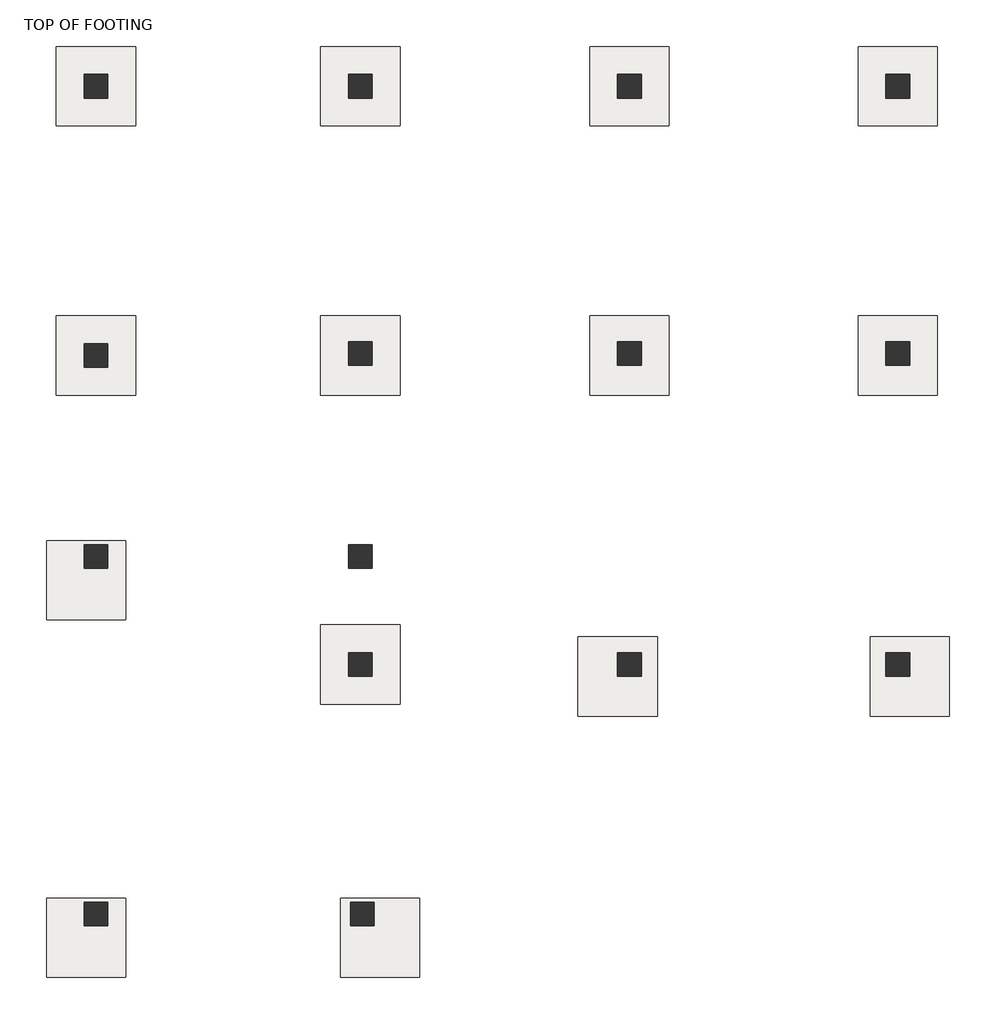
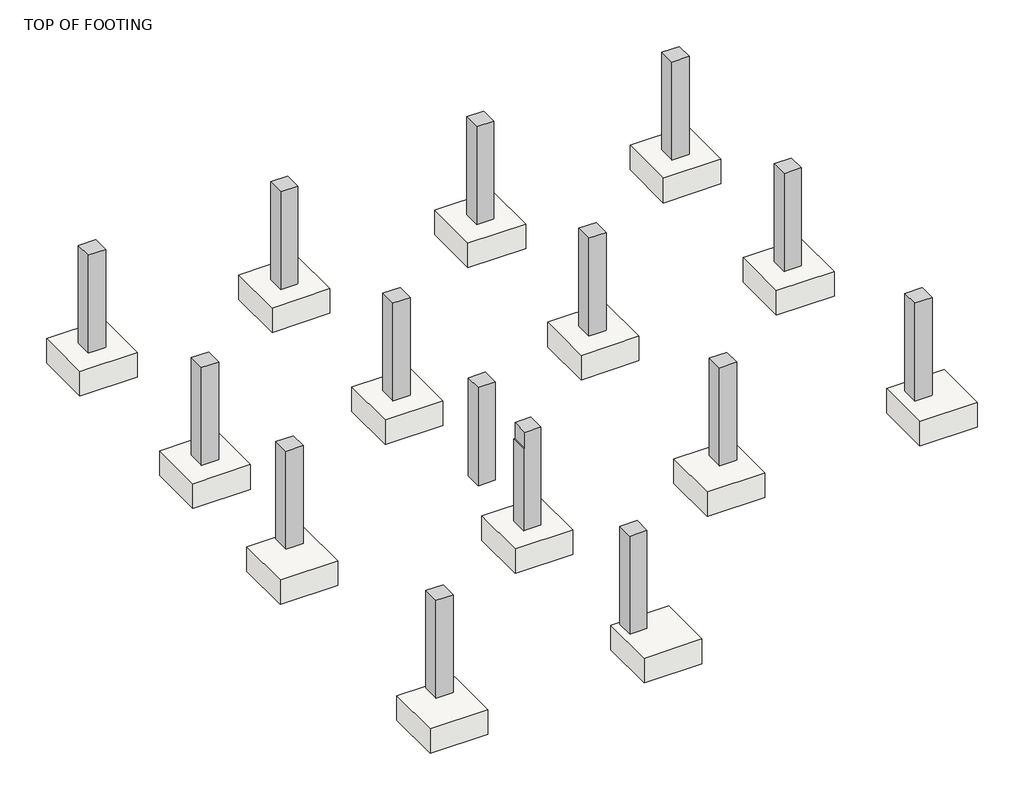
# One storey: 15 columns, 14 slabs.
"""IFC4 building model written with IfcOpenShell, lengths in millimetres."""

from ifc_helpers import new_model, si_unit, frame, origin, place, context, project, spatial, polyline, outline, extrude, faceted_brep, transform, mapped, element, save
from components import slab_21579c01

model = new_model("IFC4")

# Units and contexts
model_context = context("Model", 3, world=origin())
ifc_project = project(units=[si_unit("LENGTHUNIT", "METRE", prefix="MILLI")], contexts=[model_context])

# Site, building, storey
site = spatial("IfcSite", under=ifc_project)
building = spatial("IfcBuilding", under=site)
storey = spatial("IfcBuildingStorey", under=building, Name="TOP OF FOOTING", Elevation=-1828.8)

# Columns
placement = place(None, origin())
element("IfcColumn", 1, ObjectType="Concrete-Rectangular-Column : 12\" X 12\" COLUMN", at=placement, inside=storey, context=model_context, shape_type="SweptSolid", body=[
    extrude(outline(polyline([(-11339.0293601, -2564.0747117), (-11339.0293601, -2868.8747117), (-11643.8293601, -2868.8747117), (-11643.8293601, -2564.0747117), (-11339.0293601, -2564.0747117)])), frame((0.0, 0.0, -1828.8), z_axis=(0.0, 0.0, 1.0), x_axis=(1.0, 0.0, 0.0)), (0.0, 0.0, 1.0), 1828.8),
])
element("IfcColumn", 2, ObjectType="Concrete-Rectangular-Column : 12\" X 12\" COLUMN", at=placement, inside=storey, context=model_context, shape_type="SweptSolid", body=[
    extrude(outline(polyline([(-7946.7270642, -2564.0747117), (-7946.7270642, -2868.8747117), (-8251.5270642, -2868.8747117), (-8251.5270642, -2564.0747117), (-7946.7270642, -2564.0747117)])), frame((0.0, 0.0, -1828.8), z_axis=(0.0, 0.0, 1.0), x_axis=(1.0, 0.0, 0.0)), (0.0, 0.0, 1.0), 1828.8),
])
element("IfcColumn", 3, ObjectType="Concrete-Rectangular-Column : 12\" X 12\" COLUMN", at=placement, inside=storey, context=model_context, shape_type="SweptSolid", body=[
    extrude(outline(polyline([(-4492.3270642, -2564.0747117), (-4492.3270642, -2868.8747117), (-4797.1270642, -2868.8747117), (-4797.1270642, -2564.0747117), (-4492.3270642, -2564.0747117)])), frame((0.0, 0.0, -1828.8), z_axis=(0.0, 0.0, 1.0), x_axis=(1.0, 0.0, 0.0)), (0.0, 0.0, 1.0), 1828.8),
])
element("IfcColumn", 4, ObjectType="Concrete-Rectangular-Column : 12\" X 12\" COLUMN", at=placement, inside=storey, context=model_context, shape_type="SweptSolid", body=[
    extrude(outline(polyline([(-1047.1658472, -2564.0747117), (-1047.1658472, -2868.8747117), (-1351.9658472, -2868.8747117), (-1351.9658472, -2564.0747117), (-1047.1658472, -2564.0747117)])), frame((0.0, 0.0, -1828.8), z_axis=(0.0, 0.0, 1.0), x_axis=(1.0, 0.0, 0.0)), (0.0, 0.0, 1.0), 1828.8),
])
element("IfcColumn", 5, ObjectType="Concrete-Rectangular-Column : 12\" X 12\" COLUMN", at=placement, inside=storey, context=model_context, shape_type="SweptSolid", body=[
    extrude(outline(polyline([(-1047.1658472, -5993.0747117), (-1047.1658472, -6297.8747117), (-1351.9658472, -6297.8747117), (-1351.9658472, -5993.0747117), (-1047.1658472, -5993.0747117)])), frame((0.0, 0.0, -1828.8), z_axis=(0.0, 0.0, 1.0), x_axis=(1.0, 0.0, 0.0)), (0.0, 0.0, 1.0), 1828.8),
])
element("IfcColumn", 6, ObjectType="Concrete-Rectangular-Column : 12\" X 12\" COLUMN", at=placement, inside=storey, context=model_context, shape_type="SweptSolid", body=[
    extrude(outline(polyline([(-4492.3270642, -5993.0747117), (-4492.3270642, -6297.8747117), (-4797.1270642, -6297.8747117), (-4797.1270642, -5993.0747117), (-4492.3270642, -5993.0747117)])), frame((0.0, 0.0, -1828.8), z_axis=(0.0, 0.0, 1.0), x_axis=(1.0, 0.0, 0.0)), (0.0, 0.0, 1.0), 1828.8),
])
element("IfcColumn", 7, ObjectType="Concrete-Rectangular-Column : 12\" X 12\" COLUMN", at=placement, inside=storey, context=model_context, shape_type="Brep", body=[
    faceted_brep([(-7946.7270642, -5993.0747117, -1828.8), (-7946.7270642, -6297.8747117, -1828.8), (-8251.5270642, -6297.8747117, -1828.8), (-8251.5270642, -5993.0747117, -1828.8), (-7946.7270642, -5993.0747117, 0.0), (-7946.7270642, -6297.8747117, 0.0), (-8251.5270642, -6297.8747117, 0.0), (-8251.5270642, -6018.4747117, 0.0), (-8251.5270642, -5993.0747117, 0.0)], [[[0, 1, 2, 3]], [[4, 5, 1, 0]], [[5, 6, 2, 1]], [[6, 7, 8, 3, 2]], [[8, 4, 0, 3]], [[4, 8, 7, 6, 5]]]),
])
element("IfcColumn", 8, ObjectType="Concrete-Rectangular-Column : 12\" X 12\" COLUMN", at=placement, inside=storey, context=model_context, shape_type="SweptSolid", body=[
    extrude(outline(polyline([(-11339.0293601, -6018.4747117), (-11339.0293601, -6323.2747117), (-11643.8293601, -6323.2747117), (-11643.8293601, -6018.4747117), (-11339.0293601, -6018.4747117)])), frame((0.0, 0.0, -1828.8), z_axis=(0.0, 0.0, 1.0), x_axis=(1.0, 0.0, 0.0)), (0.0, 0.0, 1.0), 1828.8),
])
element("IfcColumn", 9, ObjectType="Concrete-Rectangular-Column : 12\" X 12\" COLUMN", at=placement, inside=storey, context=model_context, shape_type="SweptSolid", body=[
    extrude(outline(polyline([(-11339.0293601, -8597.9373391), (-11339.0293601, -8902.7373391), (-11643.8293601, -8902.7373391), (-11643.8293601, -8597.9373391), (-11339.0293601, -8597.9373391)])), frame((0.0, 0.0, -1828.8), z_axis=(0.0, 0.0, 1.0), x_axis=(1.0, 0.0, 0.0)), (0.0, 0.0, 1.0), 1828.8),
])
element("IfcColumn", 10, ObjectType="Concrete-Rectangular-Column : 12\" X 12\" COLUMN", at=placement, inside=storey, context=model_context, shape_type="SweptSolid", body=[
    extrude(outline(polyline([(-7946.7270642, -8597.9373391), (-7946.7270642, -8902.7373391), (-8251.5270642, -8902.7373391), (-8251.5270642, -8597.9373391), (-7946.7270642, -8597.9373391)])), frame((0.0, 0.0, -1828.8), z_axis=(0.0, 0.0, 1.0), x_axis=(1.0, 0.0, 0.0)), (0.0, 0.0, 1.0), 1828.8),
])
element("IfcColumn", 11, ObjectType="Concrete-Rectangular-Column : 12\" X 12\" COLUMN", at=placement, inside=storey, context=model_context, shape_type="Brep", body=[
    faceted_brep([(-7921.3270642, -13183.002305, -1828.8), (-7921.3270642, -13487.802305, -1828.8), (-8226.1270642, -13487.802305, -1828.8), (-8226.1270642, -13183.002305, -1828.8), (-7921.3270642, -13183.002305, 0.0), (-7921.3270642, -13487.802305, 0.0), (-8226.1270642, -13487.802305, 0.0), (-8226.1270642, -13487.802305, -304.8), (-8226.1270642, -13183.002305, 0.0), (-8226.1270642, -13183.002305, -304.8)], [[[0, 1, 2, 3]], [[4, 5, 1, 0]], [[5, 6, 7, 2, 1]], [[6, 8, 9, 3, 2, 7]], [[8, 4, 0, 3, 9]], [[4, 8, 6, 5]]]),
])
element("IfcColumn", 12, ObjectType="Concrete-Rectangular-Column : 12\" X 12\" COLUMN", at=placement, inside=storey, context=model_context, shape_type="Brep", body=[
    faceted_brep([(-11339.0293601, -13183.002305, -1828.8), (-11339.0293601, -13487.802305, -1828.8), (-11643.8293601, -13487.802305, -1828.8), (-11643.8293601, -13183.002305, -1828.8), (-11339.0293601, -13183.002305, 0.0), (-11339.0293601, -13487.802305, 0.0), (-11339.0293601, -13487.802305, -304.8), (-11339.0293601, -13183.002305, -304.8), (-11643.8293601, -13487.802305, 0.0), (-11643.8293601, -13183.002305, 0.0)], [[[0, 1, 2, 3]], [[4, 5, 6, 1, 0, 7]], [[5, 8, 2, 1, 6]], [[8, 9, 3, 2]], [[9, 4, 7, 0, 3]], [[4, 9, 8, 5]]]),
])
element("IfcColumn", 13, ObjectType="Concrete-Rectangular-Column : 12\" X 12\" COLUMN", at=placement, inside=storey, context=model_context, shape_type="SweptSolid", body=[
    extrude(outline(polyline([(-1828.8, -8251.5270642), (-1828.8, -7946.7270642), (0.0, -7946.7270642), (0.0, -8226.1270642), (-304.8, -8226.1270642), (-304.8, -8251.5270642), (-1828.8, -8251.5270642)])), frame((0.0, -10288.8050402, 0.0), z_axis=(0.0, 1.0, 0.0), x_axis=(0.0, 0.0, 1.0)), (0.0, 0.0, 1.0), 304.8),
])
element("IfcColumn", 14, ObjectType="Concrete-Rectangular-Column : 12\" X 12\" COLUMN", at=placement, inside=storey, context=model_context, shape_type="SweptSolid", body=[
    extrude(outline(polyline([(-4492.3270642, -9984.0050402), (-4492.3270642, -10288.8050402), (-4797.1270642, -10288.8050402), (-4797.1270642, -9984.0050402), (-4492.3270642, -9984.0050402)])), frame((0.0, 0.0, -1828.8), z_axis=(0.0, 0.0, 1.0), x_axis=(1.0, 0.0, 0.0)), (0.0, 0.0, 1.0), 1828.8),
])
element("IfcColumn", 15, ObjectType="Concrete-Rectangular-Column : 12\" X 12\" COLUMN", at=placement, inside=storey, context=model_context, shape_type="SweptSolid", body=[
    extrude(outline(polyline([(-1047.1658472, -9984.0050402), (-1047.1658472, -10288.8050402), (-1351.9658472, -10288.8050402), (-1351.9658472, -9984.0050402), (-1047.1658472, -9984.0050402)])), frame((0.0, 0.0, -1828.8), z_axis=(0.0, 0.0, 1.0), x_axis=(1.0, 0.0, 0.0)), (0.0, 0.0, 1.0), 1828.8),
])

# Slabs
slab_shape = slab_21579c01(model_context)
element("IfcSlab", 16, ObjectType="Footing-Rectangular : 40\" X 40\" X18\"", at=placement, inside=storey, context=model_context, shape_type="MappedRepresentation", body=[
    mapped(slab_shape, transform((-11618.4293601, -9055.1373391, -1828.8), x_axis=(1.0, 0.0, 0.0), y_axis=(0.0, 1.0, 0.0), z_axis=(0.0, 0.0, 1.0))),
])
element("IfcSlab", 17, ObjectType="Footing-Rectangular : 40\" X 40\" X18\"", at=placement, inside=storey, context=model_context, shape_type="MappedRepresentation", body=[
    mapped(slab_shape, transform((-4797.1270642, -10288.8050402, -1828.8), x_axis=(1.0, 0.0, 0.0), y_axis=(0.0, 1.0, 0.0), z_axis=(0.0, 0.0, 1.0))),
])
element("IfcSlab", 18, ObjectType="Footing-Rectangular : 40\" X 40\" X18\"", at=placement, inside=storey, context=model_context, shape_type="MappedRepresentation", body=[
    mapped(slab_shape, transform((-1047.1658472, -10288.8050402, -1828.8), x_axis=(1.0, 0.0, 0.0), y_axis=(0.0, 1.0, 0.0), z_axis=(0.0, 0.0, 1.0))),
])
element("IfcSlab", 19, ObjectType="Footing-Rectangular : 40\" X 40\" X18\"", at=placement, inside=storey, context=model_context, shape_type="MappedRepresentation", body=[
    mapped(slab_shape, transform((-11491.4293601, -2716.4747117, -1828.8), x_axis=(1.0, 0.0, 0.0), y_axis=(0.0, 1.0, 0.0), z_axis=(0.0, 0.0, 1.0))),
])
element("IfcSlab", 20, ObjectType="Footing-Rectangular : 40\" X 40\" X18\"", at=placement, inside=storey, context=model_context, shape_type="MappedRepresentation", body=[
    mapped(slab_shape, transform((-8099.1270642, -2716.4747117, -1828.8), x_axis=(1.0, 0.0, 0.0), y_axis=(0.0, 1.0, 0.0), z_axis=(0.0, 0.0, 1.0))),
])
element("IfcSlab", 21, ObjectType="Footing-Rectangular : 40\" X 40\" X18\"", at=placement, inside=storey, context=model_context, shape_type="MappedRepresentation", body=[
    mapped(slab_shape, transform((-4644.7270642, -2716.4747117, -1828.8), x_axis=(1.0, 0.0, 0.0), y_axis=(0.0, 1.0, 0.0), z_axis=(0.0, 0.0, 1.0))),
])
element("IfcSlab", 22, ObjectType="Footing-Rectangular : 40\" X 40\" X18\"", at=placement, inside=storey, context=model_context, shape_type="MappedRepresentation", body=[
    mapped(slab_shape, transform((-1199.5658472, -2716.4747117, -1828.8), x_axis=(1.0, 0.0, 0.0), y_axis=(0.0, 1.0, 0.0), z_axis=(0.0, 0.0, 1.0))),
])
element("IfcSlab", 23, ObjectType="Footing-Rectangular : 40\" X 40\" X18\"", at=placement, inside=storey, context=model_context, shape_type="MappedRepresentation", body=[
    mapped(slab_shape, transform((-11491.4293601, -6170.8747117, -1828.8), x_axis=(1.0, 0.0, 0.0), y_axis=(0.0, 1.0, 0.0), z_axis=(0.0, 0.0, 1.0))),
])
element("IfcSlab", 24, ObjectType="Footing-Rectangular : 40\" X 40\" X18\"", at=placement, inside=storey, context=model_context, shape_type="MappedRepresentation", body=[
    mapped(slab_shape, transform((-8099.1270642, -6170.8747117, -1828.8), x_axis=(1.0, 0.0, 0.0), y_axis=(0.0, 1.0, 0.0), z_axis=(0.0, 0.0, 1.0))),
])
element("IfcSlab", 25, ObjectType="Footing-Rectangular : 40\" X 40\" X18\"", at=placement, inside=storey, context=model_context, shape_type="MappedRepresentation", body=[
    mapped(slab_shape, transform((-4644.7270642, -6170.8747117, -1828.8), x_axis=(1.0, 0.0, 0.0), y_axis=(0.0, 1.0, 0.0), z_axis=(0.0, 0.0, 1.0))),
])
element("IfcSlab", 26, ObjectType="Footing-Rectangular : 40\" X 40\" X18\"", at=placement, inside=storey, context=model_context, shape_type="MappedRepresentation", body=[
    mapped(slab_shape, transform((-1199.5658472, -6170.8747117, -1828.8), x_axis=(1.0, 0.0, 0.0), y_axis=(0.0, 1.0, 0.0), z_axis=(0.0, 0.0, 1.0))),
])
element("IfcSlab", 27, ObjectType="Footing-Rectangular : 40\" X 40\" X18\"", at=placement, inside=storey, context=model_context, shape_type="MappedRepresentation", body=[
    mapped(slab_shape, transform((-8099.1270642, -10136.4050402, -1828.8), x_axis=(1.0, 0.0, 0.0), y_axis=(0.0, 1.0, 0.0), z_axis=(0.0, 0.0, 1.0))),
])
element("IfcSlab", 28, ObjectType="Footing-Rectangular : 40\" X 40\" X18\"", at=placement, inside=storey, context=model_context, shape_type="MappedRepresentation", body=[
    mapped(slab_shape, transform((-11618.4293601, -13641.6050402, -1828.8), x_axis=(1.0, 0.0, 0.0), y_axis=(0.0, 1.0, 0.0), z_axis=(0.0, 0.0, 1.0))),
])
element("IfcSlab", 29, ObjectType="Footing-Rectangular : 40\" X 40\" X18\"", at=placement, inside=storey, context=model_context, shape_type="MappedRepresentation", body=[
    mapped(slab_shape, transform((-7845.1270642, -13641.6050402, -1828.8), x_axis=(1.0, 0.0, 0.0), y_axis=(0.0, 1.0, 0.0), z_axis=(0.0, 0.0, 1.0))),
])

save(model, "model.ifc")

# Revit data of these elements
# Grids (mm)
#   "1": line (-11491.429, -16098.576) -> (-11491.429, -117.535)
#   "2": line (-8099.127, -16098.576) -> (-8099.127, -117.535)
#   "3": line (-4644.727, -16098.576) -> (-4644.727, -117.535)
#   "4": line (-1199.566, -16310.031) -> (-1199.566, -117.535)
#   "A": line (-156.36, -2716.475) -> (-13201.839, -2716.475)
#   "B": line (-156.36, -6170.875) -> (-13201.839, -6170.875)
#   "C": line (-156.36, -8750.337) -> (-12764.762, -8750.337)
# Type "Concrete-Rectangular-Column : 12\" X 12\" COLUMN"
#   Assembly Code = "B10"
#   b = 1' - 0"
#   h = 1' - 0"
#   Structural Material [instance default] = Concrete, Cast-in-Place gray
# Type "Footing-Rectangular : 40\" X 40\" X18\""
#   Assembly Code = "A1010100"
#   Width = 3' - 4"
#   Length = 3' - 4"
#   Foundation Thickness = 1' - 6"
#   Structural Material [instance default] = Concrete, Cast-in-Place gray
# Elements 1, 2, 3, 4, 5, 6, 7, 8, 9, 10, 11, 12, 13, 14, 15 (IfcColumn, "Concrete-Rectangular-Column : 12\" X 12\" COLUMN")
#   Structural Material = Concrete, Cast-in-Place gray
#   Phase Created = New Construction
#   Materials on its faces: "Concrete, Cast-in-Place gray"
# Elements 16, 17, 18, 19, 20, 21, 22, 23, 24, 25, 26, 27, 28, 29 (IfcSlab, "Footing-Rectangular : 40\" X 40\" X18\"")
#   Structural Material = Concrete, Cast-in-Place gray
#   Phase Created = New Construction
#   Materials on its faces: "Concrete, Cast-in-Place gray"
# Materials
#   "Concrete, Cast-in-Place gray": class "Concrete", colour RGB 192 192 192, transparency 0, Description = "Cast-in-place concrete", Cost = 0
